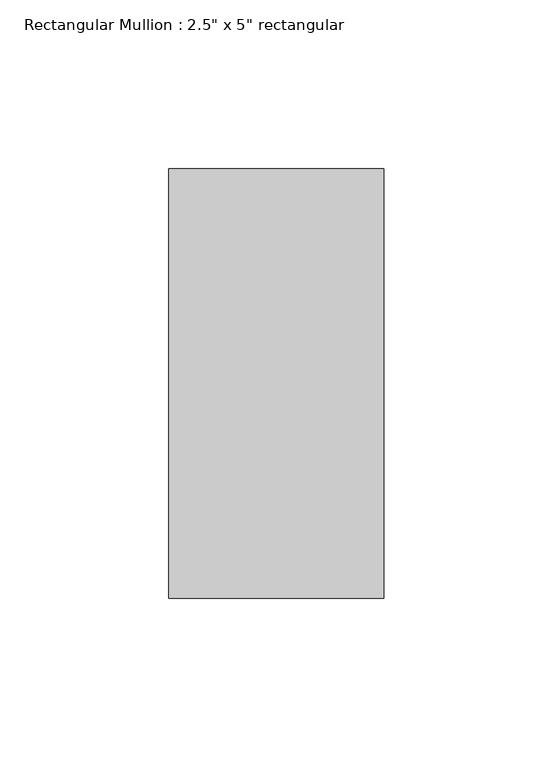
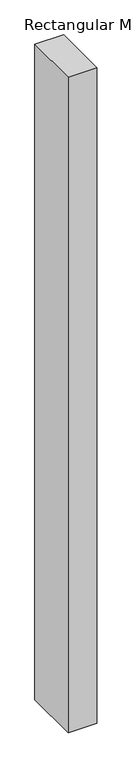
"""IFC4 building model written with IfcOpenShell, lengths in millimetres: member geometry."""

from ifc_helpers import new_model, si_unit, frame, origin, place, context, project, spatial, polyline, outline, extrude, source, transform, mapped, element, save


def member_c39a889e(model_context):
    return source(origin(), model_context, "Body", "SweptSolid", [
        extrude(outline(polyline([(31.75, 63.5), (31.75, -63.5), (-31.75, -63.5), (-31.75, 63.5), (31.75, 63.5)])), frame((0.0, 0.0, -1532.6819), z_axis=(0.0, 0.0, 1.0), x_axis=(1.0, 0.0, 0.0)), (0.0, 0.0, 1.0), 1532.6819),
    ])


if __name__ == "__main__":
    model = new_model("IFC4")
    model_context = context("Model", 3, world=origin())
    ifc_project = project(units=[si_unit("LENGTHUNIT", "METRE", prefix="MILLI")], contexts=[model_context])
    site = spatial("IfcSite", under=ifc_project)
    building = spatial("IfcBuilding", under=site)
    placement = place(None, origin())
    member_shape = member_c39a889e(model_context)
    element("IfcMember", 1, ObjectType="Rectangular Mullion : 2.5\" x 5\" rectangular", at=placement, inside=building, context=model_context, shape_type="MappedRepresentation", body=[
        mapped(member_shape, transform((0.0, 0.0, 0.0), x_axis=(1.0, 0.0, 0.0), y_axis=(0.0, 1.0, 0.0), z_axis=(0.0, 0.0, 1.0))),
    ])
    save(model, "model.ifc")

# Revit data of these elements
# Type "Rectangular Mullion : 2.5\" x 5\" rectangular"
#   built-in parameter 1007304 = 0.416667 (stored number, unit not read)
#   built-in parameter 1007301 = 0.104167 (stored number, unit not read)
#   built-in parameter 1007300 = 0.104167 (stored number, unit not read)
# Element 1 (IfcMember, "Rectangular Mullion : 2.5\" x 5\" rectangular")
#   Materials on its faces: "Aluminum"
# Materials
#   "Aluminum": class "Metal", colour RGB 247 247 247, transparency 0, Description = "Aluminum 6061", Cost = 0
